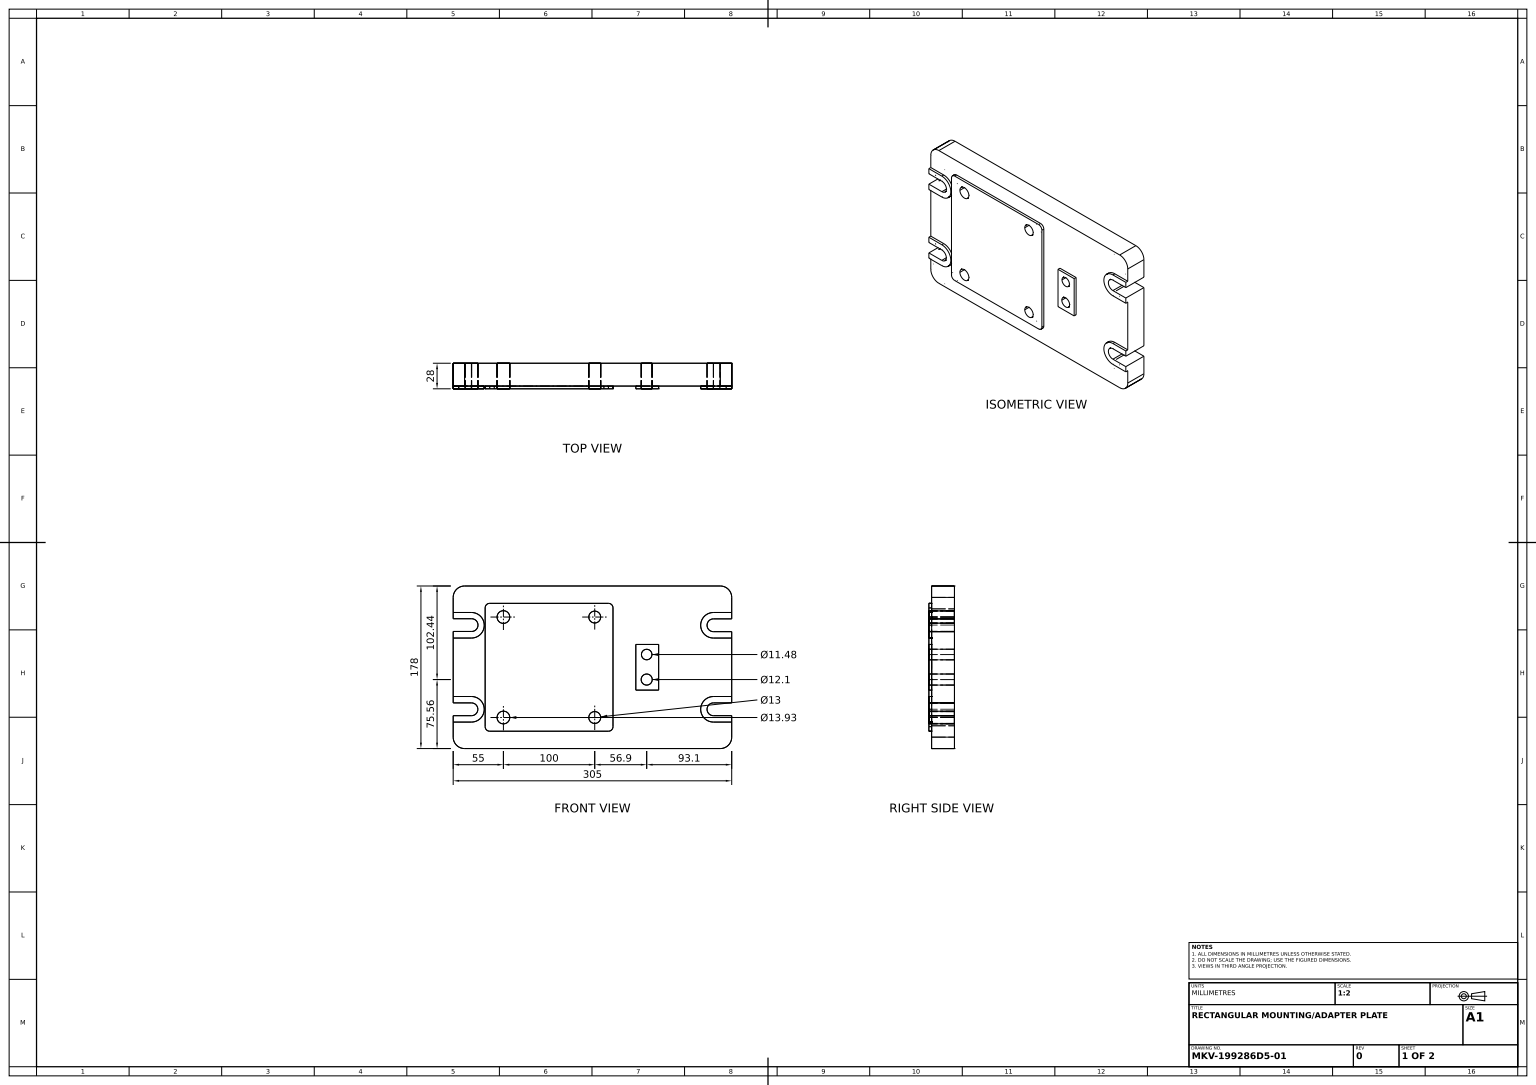
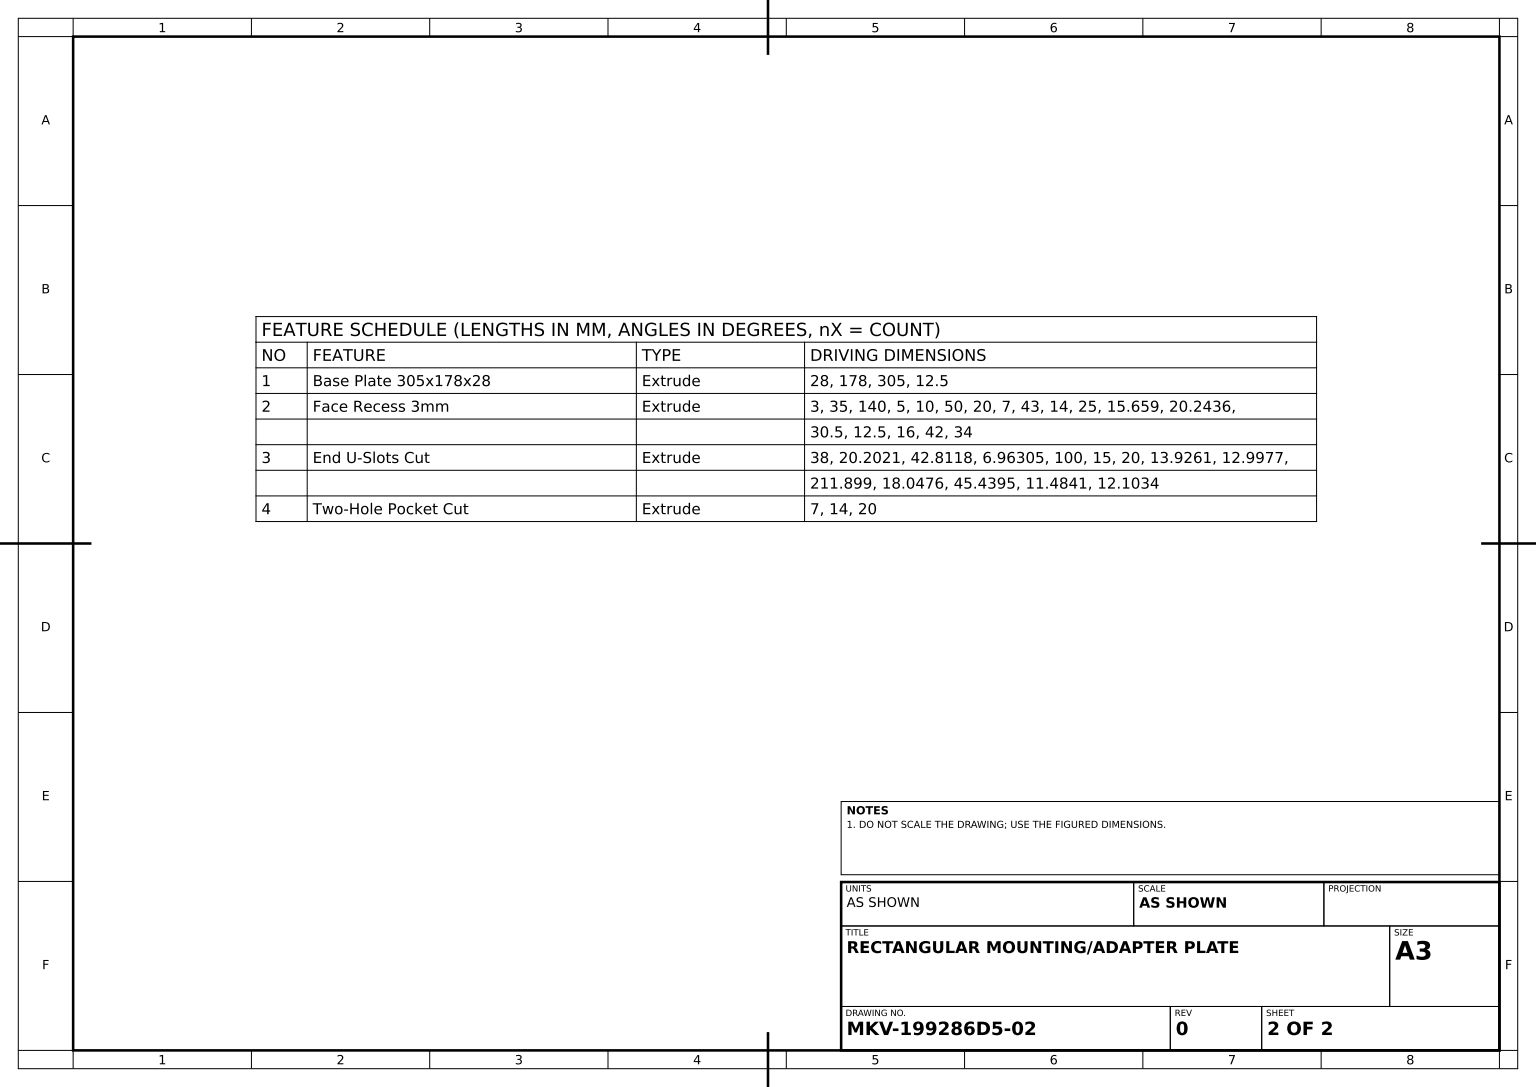
from build123d import *

# Parameters (mm, degrees)
BASE_PLATE_305X178X28_DEPTH    = 14
FACE_RECESS_3MM_DEPTH          = 3
END_SLOTS_PROFILE_R            = 6.963047248
END_SLOTS_PROFILE_R_2          = 6.498844098
END_SLOTS_PROFILE_R_3          = 5.742027746
END_SLOTS_PROFILE_R_4          = 6.051697443
END_U_SLOTS_CUT_DEPTH          = 38
TWO_HOLE_POCKET_CUT_DEPTH      = 179.777095848
TWO_HOLE_POCKET_CUT_DEPTH_BACK = 179.777095848


with BuildPart() as part:
    # Base Plate Profile → Base Plate 305x178x28 (new, symmetric)
    with BuildSketch(Plane.XY):
        with BuildLine():
            Line((-140, 89), (140, 89))
            ThreePointArc((140, 89), (148.838834765, 85.338834765), (152.5, 76.5))
            Line((152.5, 76.5), (152.5, -76.5))
            ThreePointArc((152.5, -76.5), (148.838834765, -85.338834765), (140, -89))
            Line((140, -89), (-140, -89))
            ThreePointArc((-140, -89), (-148.838834765, -85.338834765), (-152.5, -76.5))
            Line((-152.5, -76.5), (-152.5, 76.5))
            ThreePointArc((-152.5, 76.5), (-148.838834765, 85.338834765), (-140, 89))
        make_face()
    extrude(amount=BASE_PLATE_305X178X28_DEPTH, both=True)

    # Face Recess Profile → Face Recess 3mm (cut)
    with BuildSketch(Plane.XY.offset(14)):
        with BuildLine():
            ThreePointArc((-152.5, -76.5), (-148.838834765, -85.338834765), (-140, -89))
            Line((-140, -89), (140, -89))
            ThreePointArc((140, -89), (148.838834765, -85.338834765), (152.5, -76.5))
            Line((152.5, -76.5), (152.5, -60))
            Line((152.5, -60), (132.5, -60))
            ThreePointArc((132.5, -60), (118.5, -46), (132.5, -32))
            Line((132.5, -32), (152.5, -32))
            Line((152.5, -32), (152.5, 32))
            Line((152.5, 32), (132.5, 32))
            ThreePointArc((132.5, 32), (118.5, 46), (132.5, 60))
            Line((132.5, 60), (152.5, 60))
            Line((152.5, 60), (152.5, 76.5))
            ThreePointArc((152.5, 76.5), (148.838834765, 85.338834765), (140, 89))
            Line((140, 89), (-140, 89))
            ThreePointArc((-140, 89), (-148.838834765, 85.338834765), (-152.5, 76.5))
            Line((-152.5, 76.5), (-152.5, 60))
            Line((-152.5, 60), (-132.5, 60))
            ThreePointArc((-132.5, 60), (-118.5, 46), (-132.5, 32))
            Line((-132.5, 32), (-152.5, 32))
            Line((-152.5, 32), (-152.5, -32))
            Line((-152.5, -32), (-132.5, -32))
            ThreePointArc((-132.5, -32), (-118.5, -46), (-132.5, -60))
            Line((-132.5, -60), (-152.5, -60))
            Line((-152.5, -60), (-152.5, -76.5))
        make_face()
        with BuildLine():
            ThreePointArc((-117.5, 65), (-116.035533906, 68.535533906), (-112.5, 70))
            Line((-112.5, 70), (17.5, 70))
            ThreePointArc((17.5, 70), (21.035533906, 68.535533906), (22.5, 65))
            Line((22.5, 65), (22.5, -65))
            ThreePointArc((22.5, -65), (21.035533906, -68.535533906), (17.5, -70))
            Line((17.5, -70), (-112.5, -70))
            ThreePointArc((-112.5, -70), (-116.035533906, -68.535533906), (-117.5, -65))
            Line((-117.5, -65), (-117.5, 65))
        make_face(mode=Mode.SUBTRACT)
        Polygon((47.5, -25), (47.5, 25), (72.5, 25), (72.5, -25), (60, -25), align=None, mode=Mode.SUBTRACT)
    extrude(amount=-FACE_RECESS_3MM_DEPTH, mode=Mode.SUBTRACT)

    # End Slots Profile → End U-Slots Cut (cut)
    with BuildSketch(Plane.XY.offset(14)):
        with BuildLine():
            Line((-132.297897709, 53.151260658), (-152.5, 53.151260658))
            Line((-152.5, 53.151260658), (-152.5, 39.225166163))
            Line((-152.5, 39.225166163), (-132.297897709, 39.225166163))
            ThreePointArc((-132.297897709, 39.225166163), (-125.334850461, 46.188213411), (-132.297897709, 53.151260658))
        make_face()
        with Locations((-97.5, 55)):
            Circle(END_SLOTS_PROFILE_R)
        with Locations((2.5, 55)):
            Circle(END_SLOTS_PROFILE_R_2)
        with Locations((2.5, -55)):
            Circle(END_SLOTS_PROFILE_R_2)
        with Locations((59.398868635, 13.95239873)):
            Circle(END_SLOTS_PROFILE_R_3)
        with Locations((-97.5, -55)):
            Circle(END_SLOTS_PROFILE_R)
        with Locations((59.398868635, -13.43949496)):
            Circle(END_SLOTS_PROFILE_R_4)
    extrude(amount=-END_U_SLOTS_CUT_DEPTH, mode=Mode.SUBTRACT)

    # Hole Pocket Profile → Two-Hole Pocket Cut (cut, two sides: drawn at the far end of the back side and taken through both)
    with BuildSketch(Plane.XY.offset(14).offset(-TWO_HOLE_POCKET_CUT_DEPTH_BACK)):
        with BuildLine():
            Line((-152.5, -39), (-132.5, -39))
            ThreePointArc((-132.5, -39), (-125.5, -46), (-132.5, -53))
            Line((-132.5, -53), (-152.5, -53))
            Line((-152.5, -53), (-152.5, -39))
        make_face()
        with BuildLine():
            Line((152.5, -39), (152.5, -53))
            Line((152.5, -53), (132.5, -53))
            ThreePointArc((132.5, -53), (125.5, -46), (132.5, -39))
            Line((132.5, -39), (152.5, -39))
        make_face()
        with BuildLine():
            Line((152.5, 39), (132.5, 39))
            ThreePointArc((132.5, 39), (125.5, 46), (132.5, 53))
            Line((132.5, 53), (152.5, 53))
            Line((152.5, 53), (152.5, 39))
        make_face()
    extrude(amount=TWO_HOLE_POCKET_CUT_DEPTH + TWO_HOLE_POCKET_CUT_DEPTH_BACK, mode=Mode.SUBTRACT)


solid = part.part
